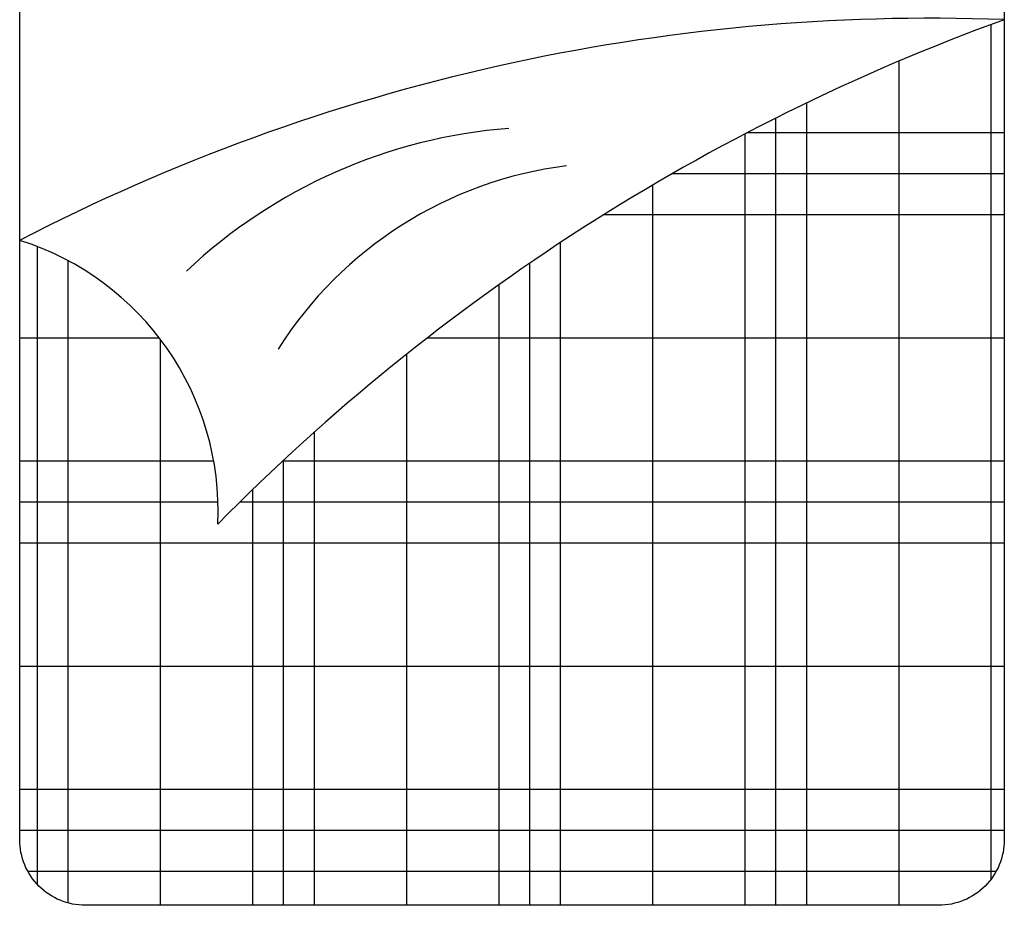
# Model space of a CAD drawing. Units: inches. Extents: x 3064 to 19385, y 846 to 15425.
# Tile 31 of 108: x 4973 to 5033, y 1315 to 1368. Entities that reach past the tile are written whole.
import ezdxf

# ---------------------------------------------------------------- set-up
doc = ezdxf.new("R2010")
doc.units = ezdxf.units.IN
doc.layers.add('A-FLOR-FIXT', color=9, linetype='Continuous', lineweight=18)
doc.layers.add('BLOCK', color=6, linetype='Continuous')

# ---------------------------------------------------------------- blocks, each defined once
blk = doc.blocks.new('*X5')
at = {"color": 0}
for p, q in [((276.598, 451.25), (280.51, 451.25)), ((275.455, 450.625), (280.51, 450.625)), ((274.411, 450), (280.51, 450)), ((265.51, 448.125), (267.634, 448.125)), ((271.723, 448.125), (280.51, 448.125)), ((265.51, 446.25), (268.465, 446.25)), ((269.519, 446.25), (280.51, 446.25)), ((265.51, 445.625), (268.531, 445.625)), ((268.866, 445.625), (280.51, 445.625)), ((265.51, 445), (280.51, 445)), ((265.51, 443.125), (280.51, 443.125)), ((265.51, 441.25), (280.51, 441.25)), ((265.51, 440.625), (280.51, 440.625)), ((265.634, 440), (280.386, 440))]:
    blk.add_line(p, q, dxfattribs=at)
blk = doc.blocks.new('*X6')
at = {"color": 0}
for p, q in [((280.312, 439.886), (280.312, 452.896)), ((278.906, 439.482), (278.906, 452.338)), ((277.5, 439.482), (277.5, 451.702)), ((277.031, 439.482), (277.031, 451.471)), ((276.562, 439.482), (276.562, 451.231)), ((275.156, 439.482), (275.156, 450.451)), ((273.75, 439.482), (273.75, 449.576)), ((265.781, 439.797), (265.781, 449.511)), ((266.25, 439.517), (266.25, 449.296)), ((273.281, 439.482), (273.281, 449.261)), ((272.812, 439.482), (272.812, 448.934)), ((267.656, 439.482), (267.656, 448.095)), ((271.406, 439.482), (271.406, 447.876)), ((270, 439.482), (270, 446.689)), ((269.531, 439.482), (269.531, 446.262)), ((269.062, 439.482), (269.062, 445.817))]:
    blk.add_line(p, q, dxfattribs=at)
blk = doc.blocks.new('A$C52E67D0D')
at = {"layer": 'BLOCK'}
blk.add_lwpolyline([(1901, 0), (601, 0, -0.414214), (501, 100), (501, 1700, -0.414214), (601, 1800), (1901, 1800, -0.414214), (2001, 1700), (2001, 100, -0.414214)], format="xyb", close=True, dxfattribs=at)
for centre, radius, start, end in [((1888.6, -1664.5), 3015.3, 87.8642, 117.4001), ((3101, -1685.8), 3227.7, 109.926, 135.3977), ((1308.8, 377.9), 807.6, 94.4436, 133.2788), ((1410.8, 520.2), 610.8, 97.2157, 147.6656), ((371.4, 600.4), 432, 357.3792, 72.5379)]:
    blk.add_arc(centre, radius, start, end, dxfattribs=at)
at = {"layer": 'BLOCK', "xscale": 100, "yscale": 100, "zscale": 100}
for name in ['*X6', '*X5']:
    blk.add_blockref(name, (-26050, -43948.2), dxfattribs=at)

msp = doc.modelspace()

# ---------------------------------------------------------------- block references
at = {"layer": 'A-FLOR-FIXT', "xscale": 0.039370099999992, "yscale": 0.039370099999992, "zscale": 0.039370099999992}
msp.add_blockref('A$C52E67D0D', (4953.724, 1315.23), dxfattribs=at)

doc.saveas('drawing.dxf')
